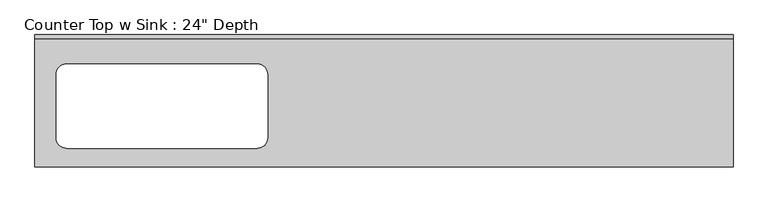
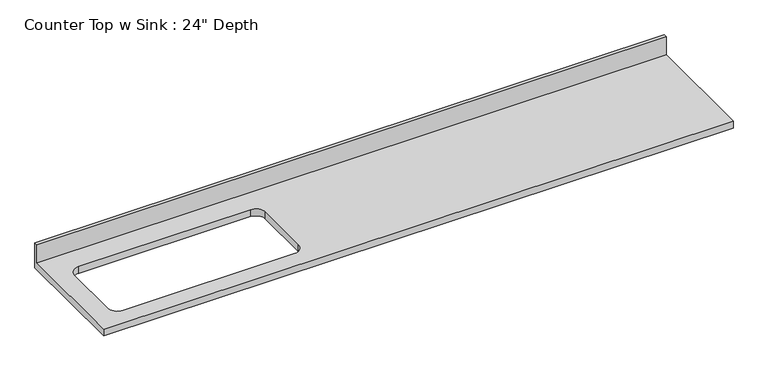
"""IFC4 building model written with IfcOpenShell, lengths in millimetres: furniture geometry."""

from ifc_helpers import new_model, si_unit, frame, origin, place, context, project, spatial, polyline, circle_curve, source, transform, mapped, element, save
from ifc_brep_helpers import plane_surface, revolved_surface, advanced_brep


def furniture_e3ff1115(model_context):
    return source(origin(), model_context, "Body", "AdvancedBrep", [
        advanced_brep(
        [(-1200.4622951, -635.0, 914.4), (2152.3377049, -635.0, 914.4), (2152.3377049, -19.05, 914.4), (-1200.4622951, -19.05, 914.4), (-1048.0622951, -139.7, 914.4), (-133.6622951, -139.7, 914.4), (-82.8622951, -190.5, 914.4), (-82.8622951, -495.3, 914.4), (-133.6622951, -546.1, 914.4), (-1048.0622951, -546.1, 914.4), (-1098.8622951, -495.3, 914.4), (-1098.8622951, -190.5, 914.4), (2152.3377049, 0.0, 876.3), (2152.3377049, -635.0, 876.3), (-1200.4622951, -635.0, 876.3), (-1200.4622951, 0.0, 876.3), (-133.6622951, -139.7, 876.3), (-1048.0622951, -139.7, 876.3), (-1098.8622951, -190.5, 876.3), (-1098.8622951, -495.3, 876.3), (-1048.0622951, -546.1, 876.3), (-133.6622951, -546.1, 876.3), (-82.8622951, -495.3, 876.3), (-82.8622951, -190.5, 876.3), (-1200.4622951, 0.0, 1016.0), (2152.3377049, 0.0, 1016.0), (-1200.4622951, -19.05, 1016.0), (2152.3377049, -19.05, 1016.0)],
        [
            (0, 1),
            (1, 2),
            (2, 3),
            (3, 0),
            (4, 5),
            (5, 6, circle_curve(frame((-133.6622951, -190.5, 914.4), z_axis=(0.0, 0.0, -1.0), x_axis=(1.0, 0.0, 0.0)), 50.8)),
            (6, 7),
            (7, 8, circle_curve(frame((-133.6622951, -495.3, 914.4), z_axis=(0.0, 0.0, -1.0), x_axis=(1.0, 0.0, 0.0)), 50.8)),
            (8, 9),
            (9, 10, circle_curve(frame((-1048.0622951, -495.3, 914.4), z_axis=(0.0, 0.0, -1.0), x_axis=(1.0, 0.0, 0.0)), 50.8)),
            (10, 11),
            (11, 4, circle_curve(frame((-1048.0622951, -190.5, 914.4), z_axis=(0.0, 0.0, -1.0), x_axis=(1.0, 0.0, 0.0)), 50.8)),
            (12, 13),
            (13, 14),
            (14, 15),
            (15, 12),
            (16, 17),
            (17, 18, circle_curve(frame((-1048.0622951, -190.5, 876.3), z_axis=(0.0, 0.0, 1.0), x_axis=(1.0, 0.0, 0.0)), 50.8)),
            (18, 19),
            (19, 20, circle_curve(frame((-1048.0622951, -495.3, 876.3), z_axis=(0.0, 0.0, 1.0), x_axis=(1.0, 0.0, 0.0)), 50.8)),
            (20, 21),
            (21, 22, circle_curve(frame((-133.6622951, -495.3, 876.3), z_axis=(0.0, 0.0, 1.0), x_axis=(1.0, 0.0, 0.0)), 50.8)),
            (22, 23),
            (23, 16, circle_curve(frame((-133.6622951, -190.5, 876.3), z_axis=(0.0, 0.0, 1.0), x_axis=(1.0, 0.0, 0.0)), 50.8)),
            (15, 24),
            (24, 25),
            (25, 12),
            (14, 0),
            (3, 26),
            (26, 24),
            (13, 1),
            (25, 27),
            (27, 2),
            (26, 27),
            (4, 17),
            (16, 5),
            (11, 18),
            (10, 19),
            (9, 20),
            (8, 21),
            (7, 22),
            (6, 23),
        ],
        [
            plane_surface(frame((-1200.4622951, 0.0, 914.4), z_axis=(0.0, 0.0, 1.0), x_axis=(-1.0, 0.0, 0.0))),
            plane_surface(frame((-1200.4622951, 0.0, 876.3), z_axis=(0.0, 0.0, -1.0), x_axis=(1.0, 0.0, 0.0))),
            plane_surface(frame((2152.3377049, 0.0, 914.4), z_axis=(0.0, 1.0, 0.0), x_axis=(0.0, 0.0, -1.0))),
            plane_surface(frame((-1200.4622951, 0.0, 914.4), z_axis=(-1.0, 0.0, 0.0), x_axis=(0.0, 0.0, -1.0))),
            plane_surface(frame((-1200.4622951, -635.0, 914.4), z_axis=(0.0, -1.0, 0.0), x_axis=(0.0, 0.0, -1.0))),
            plane_surface(frame((2152.3377049, -635.0, 914.4), z_axis=(1.0, 0.0, 0.0), x_axis=(0.0, 0.0, -1.0))),
            plane_surface(frame((-1200.4622951, 0.0, 1016.0), z_axis=(0.0, 0.0, 1.0), x_axis=(0.0, -1.0, 0.0))),
            plane_surface(frame((-1200.4622951, -19.05, 1016.0), z_axis=(0.0, -1.0, 0.0), x_axis=(0.0, 0.0, -1.0))),
            plane_surface(frame((-133.6622951, -139.7, 914.4), z_axis=(0.0, -1.0, 0.0), x_axis=(0.0, 0.0, -1.0))),
            revolved_surface(polyline([(-997.2622951000001, -190.5, 914.4), (-997.2622951000001, -190.5, 876.3)]), (-1048.0622951, -190.5, 876.3), (0.0, 0.0, 1.0)),
            plane_surface(frame((-1098.8622951, -190.5, 914.4), z_axis=(1.0, 0.0, 0.0), x_axis=(0.0, 0.0, -1.0))),
            revolved_surface(polyline([(-997.2622951000001, -495.3, 914.4), (-997.2622951000001, -495.3, 876.3)]), (-1048.0622951, -495.3, 876.3), (0.0, 0.0, 1.0)),
            plane_surface(frame((-1048.0622951, -546.1, 914.4), z_axis=(0.0, 1.0, 0.0), x_axis=(0.0, 0.0, -1.0))),
            revolved_surface(polyline([(-82.8622951, -495.3, 914.4), (-82.8622951, -495.3, 876.3)]), (-133.6622951, -495.3, 876.3), (0.0, 0.0, 1.0)),
            plane_surface(frame((-82.8622951, -495.3, 914.4), z_axis=(-1.0, 0.0, 0.0), x_axis=(0.0, 0.0, -1.0))),
            revolved_surface(polyline([(-82.8622951, -190.5, 914.4), (-82.8622951, -190.5, 876.3)]), (-133.6622951, -190.5, 876.3), (0.0, 0.0, 1.0)),
        ],
        [
            (0, [[1, 2, 3, 4], [5, 6, 7, 8, 9, 10, 11, 12]]),
            (1, [[13, 14, 15, 16], [17, 18, 19, 20, 21, 22, 23, 24]]),
            (2, [[-16, 25, 26, 27]]),
            (3, [[-15, 28, -4, 29, 30, -25]]),
            (4, [[-1, -28, -14, 31]]),
            (5, [[-13, -27, 32, 33, -2, -31]]),
            (6, [[-30, 34, -32, -26]]),
            (7, [[-34, -29, -3, -33]]),
            (8, [[35, -17, 36, -5]]),
            (9, [[-35, -12, 37, -18]]),
            (10, [[-37, -11, 38, -19]]),
            (11, [[-38, -10, 39, -20]]),
            (12, [[-39, -9, 40, -21]]),
            (13, [[-40, -8, 41, -22]]),
            (14, [[-41, -7, 42, -23]]),
            (15, [[-36, -24, -42, -6]]),
        ],
    ),
    ])


if __name__ == "__main__":
    model = new_model("IFC4")
    model_context = context("Model", 3, world=origin())
    ifc_project = project(units=[si_unit("LENGTHUNIT", "METRE", prefix="MILLI")], contexts=[model_context])
    site = spatial("IfcSite", under=ifc_project)
    building = spatial("IfcBuilding", under=site)
    placement = place(None, origin())
    furniture_shape = furniture_e3ff1115(model_context)
    element("IfcFurniture", 1, ObjectType="Counter Top w Sink : 24\" Depth", at=placement, inside=building, context=model_context, shape_type="MappedRepresentation", body=[
        mapped(furniture_shape, transform((0.0, 0.0, 0.0), x_axis=(1.0, 0.0, 0.0), y_axis=(0.0, 1.0, 0.0), z_axis=(0.0, 0.0, 1.0))),
    ])
    save(model, "model.ifc")

# Revit data of these elements
# Type "Counter Top w Sink : 24\" Depth"
#   Assembly Code = "C1030400"
#   Counter Thickness = 0' - 1 1/2"
#   Depth = 2' - 1"
#   Height = 3' - 0"
#   Length [instance default] = 8' - 0"
#   Sink Location [instance default] = 2' - 0"
#   Sink Location To Wall [instance default] = 0' - 6"
#   Sink Opening Depth [instance default] = 1' - 3"
#   Sink Opening Width [instance default] = 3' - 3"
#   Counter Top Material = none
#   Default Elevation = 0
# Element 1 (IfcFurniture, "Counter Top w Sink : 24\" Depth")
#   Length = 11' - 0"
#   Materials on its faces: "Counter Top"
# Materials
#   "Counter Top": class "Wood", colour RGB 226 177 128, transparency 0
